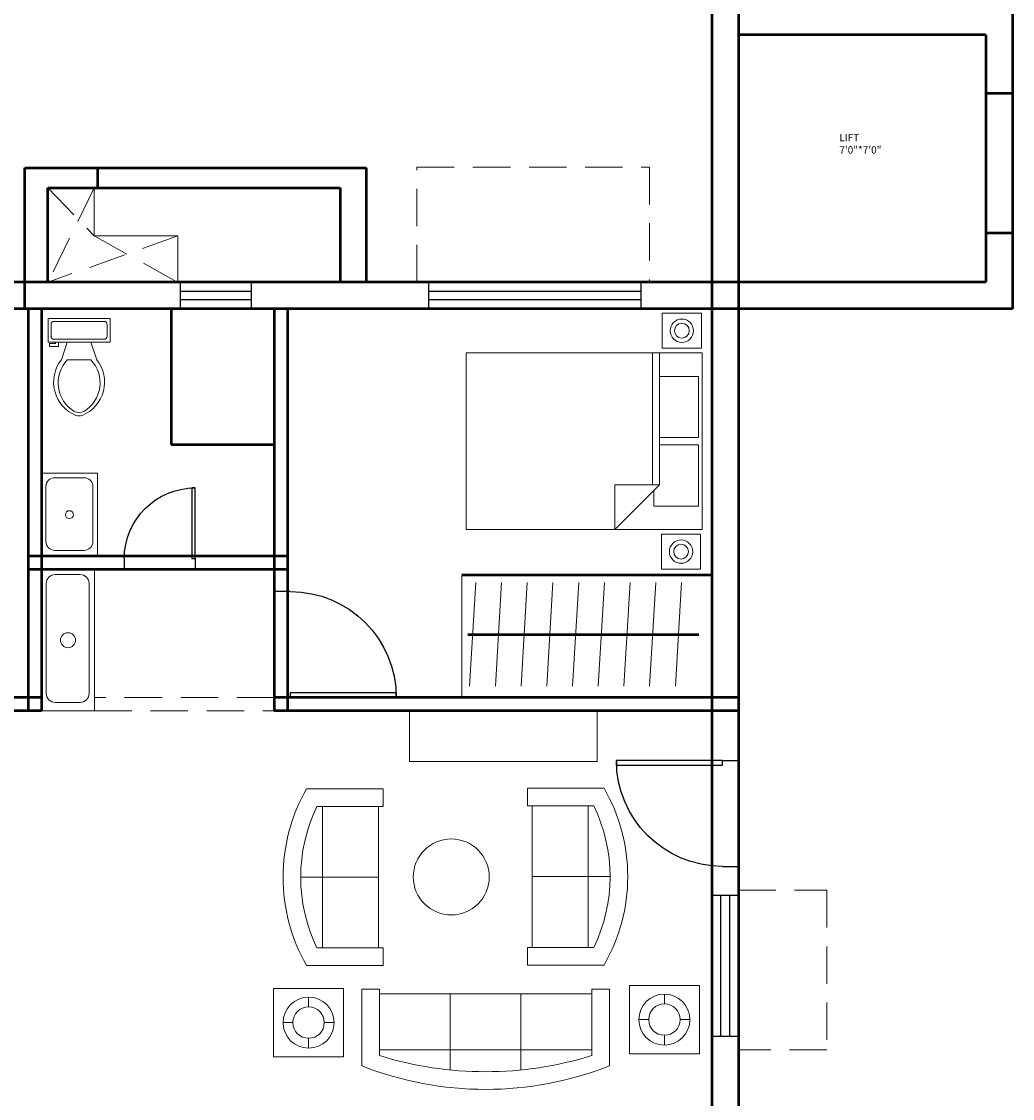
# Model space of a CAD drawing. Units: inches. Extents: x 4795 to 6024, y 2716 to 5025.
# Tile 3 of 19: x 5044 to 5380, y 2917 to 3283. Entities that reach past the tile are written whole.
import ezdxf

# ---------------------------------------------------------------- set-up
doc = ezdxf.new("R2010")
doc.units = ezdxf.units.IN
doc.linetypes.add('DASHED', pattern=[19.05, 12.7, -6.35])
for name, color, linetype, lineweight in [('A-AREA-IDEN', 3, 'Continuous', 18), ('A-DOOR', 4, 'Continuous', 25), ('A-FLOR-FIXT', 9, 'Continuous', 18), ('A-FURN', 8, 'Continuous', 18), ('A-GLAZ', 4, 'Continuous', 25), ('A-WALL', 7, 'Continuous', 50), ('A-WALL-OVHD', 8, 'DASHED', 18)]:
    doc.layers.add(name, color=color, linetype=linetype, lineweight=lineweight)
doc.styles.get("Standard").update_dxf_attribs({"font": 'arial.ttf'})

# ---------------------------------------------------------------- blocks, each defined once
blk = doc.blocks.new('*U2')
for p, q in [((0, 0), (0, -6)), ((40, 0), (40, -6))]:
    blk.add_line(p, q)
blk.add_lwpolyline([(0, 0), (0, 40), (1.75, 40), (1.75, 0)], close=True)
blk.add_arc((0, 0), 40, 0, 90)
blk = doc.blocks.new('Bed - Queen')
for p, q in [((0, -80.00003), (0, 0)), ((0, 0), (59.99999, 0)), ((59.99999, 0), (59.99999, -80.00003)), ((7.99999, -1.2), (28.79998, -1.2)), ((7.99999, -14.4), (7.99999, -1.2)), ((28.79998, -1.2), (28.79998, -14.4)), ((31.19999, -1.2), (51.99999, -1.2)), ((31.19999, -14.4), (31.19999, -1.2)), ((51.99999, -1.2), (51.99999, -16.4)), ((0, -14.4), (44.8, -14.4)), ((59.99999, -29.6), (44.8, -14.4)), ((44.8, -14.4), (44.8, -29.6)), ((44.8, -16.8), (0, -16.8)), ((51.99999, -16.4), (46.79936, -16.4)), ((44.8, -29.6), (59.99999, -29.6)), ((59.99999, -80.00003), (0, -80.00003))]:
    blk.add_line(p, q)
blk = doc.blocks.new('Sofa - Roundback 7 ft.')
for p, q in [((-12.00002, -32.4421), (-12.00003, -6.5971)), ((11.99997, -32.4421), (11.99998, -6.5971)), ((-36.000027, -34), (-36.000027, -11.4696)), ((-35.999844, -13.3819), (35.9998, -13.3819)), ((35.99998, -34), (35.99998, -11.4696)), ((-36.000027, -32.4421), (35.99998, -32.4421))]:
    blk.add_line(p, q)
for points in [[(-36.000027, -34), (-42.000027, -34), (-42.000027, -8)], [(41.99998, -8), (41.99998, -34), (35.99998, -34)]]:
    blk.add_lwpolyline(points)
for centre, radius, start, end in [((0, -114.25), 114.25, 68.43141, 111.5686), ((-0.00001, -127.1968), 121.1968, 72.72033, 107.2797)]:
    blk.add_arc(centre, radius, start, end)
blk = doc.blocks.new('Sofa - Roundback Loveseat 5 ft.')
for p, q in [((0, -32.44198), (0, -5.99998)), ((-24, -33.99998), (-24, -11.46958)), ((-23.9998, -13.38178), (23.99986, -13.38178)), ((24.00004, -33.99998), (24.00004, -11.46958)), ((-24, -32.44198), (24.00004, -32.44198))]:
    blk.add_line(p, q)
for points in [[(-24, -33.99998), (-30, -33.99998), (-30, -7.99998)], [(30.00004, -7.99998), (30.00004, -33.99998), (24.00004, -33.99998)]]:
    blk.add_lwpolyline(points)
for centre, radius, start, end in [((0, -60.24998), 60.24998, 60.13715, 119.8628), ((0, -61.38438), 55.38444, 64.32083, 115.6792)]:
    blk.add_arc(centre, radius, start, end)
blk = doc.blocks.new('Toilet - top')
for p, q in [((9.5, -6), (9.5, -2)), ((-10, -8.5), (-8, -8.5)), ((-10, -9.5), (-10, -8.5)), ((-7, -9.5), (-10, -9.5)), ((-8, -8.5), (-8, -8)), ((-7, -8), (-7, -9.5)), ((-4, -8), (-6, -14)), ((4, -8), (6, -14)), ((4, -14), (-4, -14))]:
    blk.add_line(p, q)
blk.add_lwpolyline([(10.5, -8), (10.5, 0), (-10.5, 0), (-10.5, -8)], close=True)
for points in [[(-9.5, -2), (-9.5, -6)], [(8.5, -1), (-8.5, -1)], [(-8.5, -7), (8.5, -7)]]:
    blk.add_lwpolyline(points)
for centre, radius, start, end in [((-8.62, -1.88), 0.884, 81.8699, 188.1301), ((8.62, -1.88), 0.884, 351.8699, 98.1301), ((-8.62, -6.12), 0.884, 171.8699, 278.1301), ((8.62, -6.12), 0.884, 261.8699, 8.1301), ((3.52, -21.58), 12.17, 141.4691, 247.9714), ((4.2, -21.82), 11.33, 136.3677, 238.9468), ((-3.52, -21.58), 12.17, 292.0284, 38.5307), ((-4.2, -21.82), 11.33, 301.053, 43.6321), ((0, -27.88), 4, 245.7318, 294.2682), ((0, -29), 4, 254.8605, 285.1395)]:
    blk.add_arc(centre, radius, start, end)
blk = doc.blocks.new('WIN-48')
for p, q in [((0, 0), (0, 48)), ((0, 48), (9, 48)), ((3, 0), (3, 48)), ((6, 48), (6, 0)), ((9, 48), (9, 0)), ((9, 0), (0, 0))]:
    blk.add_line(p, q)
blk = doc.blocks.new('WIN-72')
for p, q in [((0, 0), (0, 9)), ((0, 9), (72, 9)), ((72, 9), (72, 0)), ((0, 6), (72, 6)), ((72, 3), (0, 3)), ((72, 0), (0, 0))]:
    blk.add_line(p, q)
blk = doc.blocks.new('WIN-24')
for p, q in [((0, 0), (0, 9)), ((0, 9), (24, 9)), ((24, 9), (24, 0)), ((0, 6), (24, 6)), ((24, 3), (0, 3)), ((24, 0), (0, 0))]:
    blk.add_line(p, q)
blk = doc.blocks.new('LAMP-SIDE')
for p, q in [((11.88, 20.25), (11.88, 16.92)), ((3.23, 11.6), (6.56, 11.6)), ((17.2, 11.6), (20.54, 11.6)), ((11.88, 6.28), (11.88, 2.94))]:
    blk.add_line(p, q)
blk.add_lwpolyline([(23.76, 23.19), (0, 23.19), (0, 0), (23.76, 0)], close=True)
for radius in [8.66, 5.32]:
    blk.add_circle((11.88, 11.6), radius)

msp = doc.modelspace()

# ---------------------------------------------------------------- linework, layer by layer
at = {"layer": 'A-FLOR-FIXT'}
msp.add_lwpolyline([(5050.47, 3101.24), (5069.44, 3101.24), (5069.44, 3129.45), (5050.47, 3129.45)], close=True, dxfattribs=at)
msp.add_lwpolyline([(5054.96, 3127.9), (5064.89, 3127.9, -0.414214), (5067.89, 3124.9), (5067.89, 3106.23, -0.414214), (5064.89, 3103.23), (5054.96, 3103.23, -0.414214), (5051.96, 3106.23), (5051.96, 3124.9, -0.414214)], format="xyb", close=True, dxfattribs=at)
msp.add_circle((5059.95, 3115.35), 1.34, dxfattribs=at)
at = {"layer": 'A-FURN'}
for p, q in [((5068.37, 3226.31), (5068.37, 3209.95)), ((5068.37, 3209.95), (5096.69, 3209.95)), ((5096.69, 3209.95), (5096.69, 3194.24)), ((5193.16, 3053.24), (5193.16, 3094.95)), ((5195.75, 3057.14), (5197.85, 3092.27)), ((5204.48, 3057.14), (5206.58, 3092.27)), ((5213.2, 3057.14), (5215.31, 3092.27)), ((5221.93, 3057.14), (5224.04, 3092.27)), ((5230.66, 3057.14), (5232.76, 3092.27)), ((5239.39, 3057.14), (5241.49, 3092.27)), ((5248.12, 3057.14), (5250.22, 3092.27)), ((5256.84, 3057.14), (5258.95, 3092.27)), ((5265.57, 3057.14), (5267.68, 3092.27)), ((5175.31, 3048.74), (5175.31, 3031.58)), ((5239.04, 3031.58), (5239.04, 3048.74)), ((5175.31, 3031.58), (5239.04, 3031.58))]:
    msp.add_line(p, q, dxfattribs=at)
for points in [[(5261.14, 3183.74), (5274.42, 3183.74), (5274.42, 3171.81), (5261.14, 3171.81)], [(5260.87, 3108.74), (5274.14, 3108.74), (5274.14, 3096.81), (5260.87, 3096.81)], [(5050.47, 3096.74), (5068.42, 3096.74), (5068.42, 3048.71), (5050.47, 3048.71)]]:
    msp.add_lwpolyline(points, close=True, dxfattribs=at)
msp.add_lwpolyline([(5055.09, 3095.01), (5063.6, 3095.01, -0.414214), (5066.6, 3092.01), (5066.6, 3054.61, -0.414214), (5063.6, 3051.61), (5055.09, 3051.61, -0.414214), (5052.09, 3054.61), (5052.09, 3092.01, -0.414214)], format="xyb", close=True, dxfattribs=at)
for centre, radius in [((5267.78, 3177.78), 3.96), ((5267.78, 3177.78), 2.51), ((5267.51, 3102.78), 3.96), ((5267.51, 3102.78), 2.51), ((5059.45, 3072.73), 2.55), ((5189.52, 2992.36), 12.89)]:
    msp.add_circle(centre, radius, dxfattribs=at)
at = {"layer": 'A-WALL'}
for p, q in [((5277.97, 3359.43), (5277.97, 2746.24)), ((5286.97, 3350.43), (5286.97, 2746.24)), ((5379.97, 3350.43), (5379.97, 3185.24)), ((5370.97, 3278.24), (5286.97, 3278.24)), ((5370.97, 3278.24), (5370.97, 3194.24)), ((5370.97, 3258.45), (5379.97, 3258.45)), ((5044.79, 3185.24), (5044.79, 3233.1)), ((5044.79, 3233.1), (5160.66, 3233.1)), ((5069.55, 3226.31), (5069.55, 3233.1)), ((5160.66, 3233.1), (5160.66, 3194.24)), ((5052.63, 3194.24), (5052.63, 3226.31)), ((5052.63, 3226.31), (5151.81, 3226.31)), ((5151.81, 3226.31), (5151.81, 3194.24)), ((5370.97, 3210.96), (5379.97, 3210.96)), ((5286.97, 3194.24), (4892.97, 3194.24)), ((5370.97, 3194.24), (5286.97, 3194.24)), ((5286.97, 3185.24), (4901.97, 3185.24)), ((5045.97, 3185.24), (5045.97, 3048.74)), ((5050.47, 3185.24), (5050.47, 3048.74)), ((5094.47, 3185.24), (5094.47, 3139.17)), ((5129.47, 3185.24), (5129.47, 3048.74)), ((5133.97, 3185.24), (5133.97, 3048.74)), ((5379.97, 3185.24), (5286.97, 3185.24)), ((5094.47, 3139.17), (5129.47, 3139.17)), ((5133.97, 3101.24), (5045.97, 3101.24)), ((5133.97, 3096.74), (5045.97, 3096.74)), ((5193.16, 3094.95), (5277.97, 3094.95)), ((5195.12, 3074.7), (5273.55, 3074.7)), ((5050.47, 3053.24), (4892.97, 3053.24)), ((5286.97, 3053.24), (5129.47, 3053.24)), ((5050.47, 3048.74), (4892.97, 3048.74)), ((5286.97, 3048.74), (5129.47, 3048.74))]:
    msp.add_line(p, q, dxfattribs=at)
at = {"layer": 'A-WALL-OVHD'}
for p, q in [((5177.82, 3194.24), (5177.82, 3233.32)), ((5177.82, 3233.32), (5256.82, 3233.32)), ((5256.82, 3233.32), (5256.82, 3194.24)), ((5068.37, 3226.31), (5052.63, 3194.24)), ((5052.63, 3226.31), (5068.37, 3209.95)), ((5096.69, 3209.95), (5052.63, 3194.24)), ((5068.37, 3209.95), (5096.69, 3194.24)), ((5129.47, 3053.24), (5068.42, 3053.24)), ((5068.42, 3048.71), (5129.47, 3048.74)), ((5286.97, 2987.85), (5317, 2987.85)), ((5317, 2987.85), (5317, 2933.65)), ((5317, 2933.65), (5286.97, 2933.65))]:
    msp.add_line(p, q, dxfattribs=at)

# ---------------------------------------------------------------- block references
at = {"layer": 'A-DOOR', "xscale": -0.6, "yscale": 0.6, "zscale": 0.6}
msp.add_blockref('*U2', (5102.56, 3100.42), dxfattribs=at)
at = {"layer": 'A-DOOR', "xscale": -0.9, "yscale": 0.9, "zscale": 0.9}
for p, rotation in [((5134.87, 3053.24), 270), ((5281.57, 3031.93), 90)]:
    msp.add_blockref('*U2', p, dxfattribs=dict(at, rotation=rotation))
at = {"layer": 'A-FLOR-FIXT'}
msp.add_blockref('Toilet - top', (5063.21, 3181.91), dxfattribs=at)
at = {"layer": 'A-FURN'}
for name, p, rotation in [('Bed - Queen', (5274.63, 3170.28), 270), ('Sofa - Roundback Loveseat 5 ft.', (5132.43, 2992.27), 90), ('Sofa - Roundback Loveseat 5 ft.', (5249.4, 2992.46), 270), ('Sofa - Roundback 7 ft.', (5201.18, 2920.24), 180)]:
    msp.add_blockref(name, p, dxfattribs=dict(at, rotation=rotation))
for p in [(5129.24, 2931.3), (5249.96, 2932.32)]:
    msp.add_blockref('LAMP-SIDE', p, dxfattribs=at)
at = {"layer": 'A-GLAZ', "rotation": 180}
for name, p in [('WIN-24', (5121.59, 3194.24)), ('WIN-72', (5253.9, 3194.24))]:
    msp.add_blockref(name, p, dxfattribs=at)
at = {"layer": 'A-GLAZ'}
msp.add_blockref('WIN-48', (5277.97, 2938.14), dxfattribs=at)

# ---------------------------------------------------------------- texts
at = {"layer": 'A-AREA-IDEN', "insert": (5321.22, 3244.59), "char_height": 2.5, "attachment_point": 1}
msp.add_mtext_dynamic_manual_height_columns('LIFT\\P7\'0"*7\'0"', width=36.0816, gutter_width=12.5, heights=[0], dxfattribs=at)

doc.saveas('drawing.dxf')
